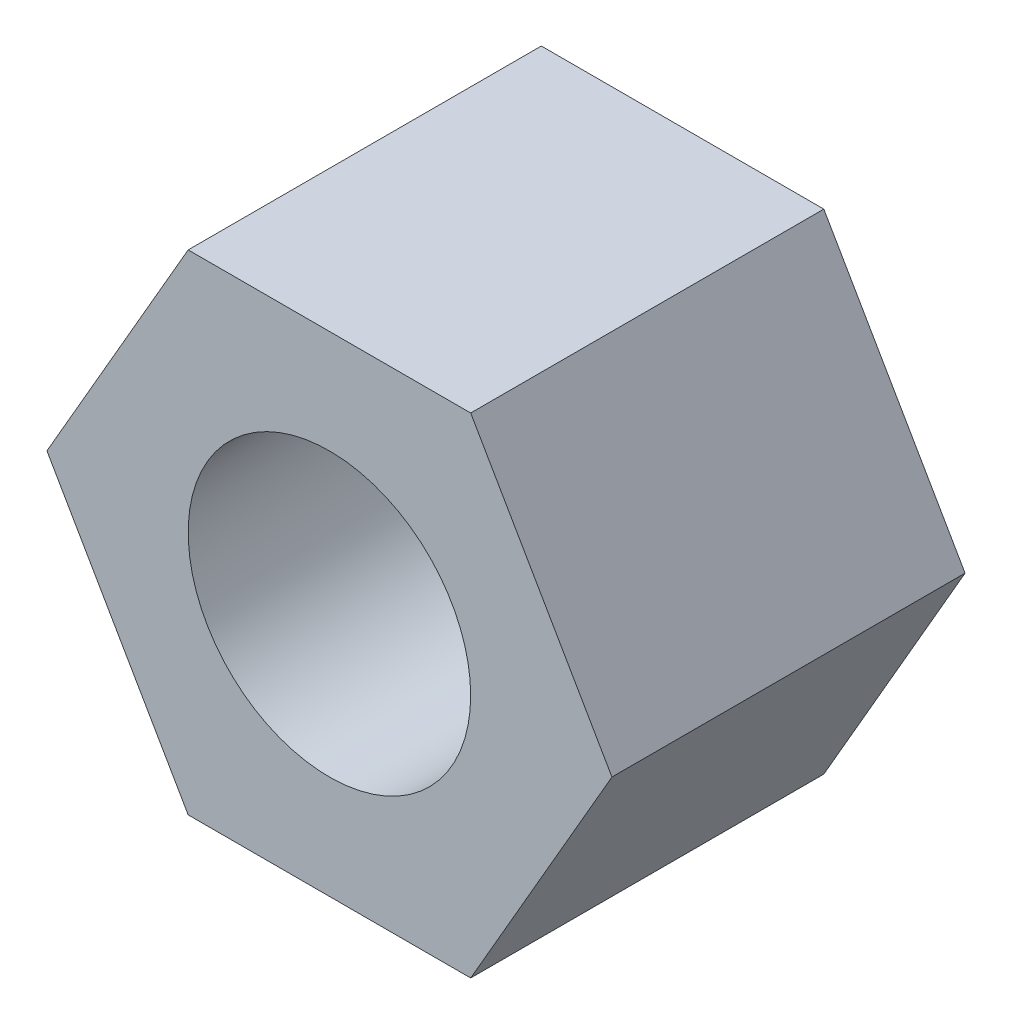
ISO-10303-21;
HEADER;
FILE_DESCRIPTION(('STEP AP214'),'2;1');
FILE_NAME('part.step','',(''),(''),'','','');
FILE_SCHEMA(('AUTOMOTIVE_DESIGN { 1 0 10303 214 1 1 1 1 }'));
ENDSEC;
DATA;
#1=APPLICATION_CONTEXT('core data for automotive mechanical design processes');
#2=APPLICATION_PROTOCOL_DEFINITION('international standard','automotive_design',2000,#1);
#3=PRODUCT_CONTEXT('',#1,'mechanical');
#4=PRODUCT('Part','Part','',(#3));
#5=PRODUCT_RELATED_PRODUCT_CATEGORY('part','',(#4));
#6=PRODUCT_DEFINITION_FORMATION('','',#4);
#7=PRODUCT_DEFINITION_CONTEXT('part definition',#1,'design');
#8=PRODUCT_DEFINITION('design','',#6,#7);
#9=PRODUCT_DEFINITION_SHAPE('','',#8);
#10=(LENGTH_UNIT() NAMED_UNIT(*) SI_UNIT(.MILLI.,.METRE.));
#11=(NAMED_UNIT(*) PLANE_ANGLE_UNIT() SI_UNIT($,.RADIAN.));
#12=(NAMED_UNIT(*) SI_UNIT($,.STERADIAN.) SOLID_ANGLE_UNIT());
#13=UNCERTAINTY_MEASURE_WITH_UNIT(LENGTH_MEASURE(1.E-05),#10,'distance_accuracy_value','');
#14=(GEOMETRIC_REPRESENTATION_CONTEXT(3) GLOBAL_UNCERTAINTY_ASSIGNED_CONTEXT((#13)) GLOBAL_UNIT_ASSIGNED_CONTEXT((#10,
#11,#12)) REPRESENTATION_CONTEXT('',''));
#15=CARTESIAN_POINT('',(0.,0.,0.));
#16=DIRECTION('',(0.,0.,1.));
#17=DIRECTION('',(1.,0.,0.));
#18=AXIS2_PLACEMENT_3D('',#15,#16,#17);
#19=CARTESIAN_POINT('',(0.,0.,15.));
#20=DIRECTION('',(0.,0.,1.));
#21=DIRECTION('',(1.,0.,0.));
#22=AXIS2_PLACEMENT_3D('',#19,#20,#21);
#23=PLANE('',#22);
#24=DIRECTION('',(0.499999999999995,0.866025403784441,0.));
#25=VECTOR('',#24,1.);
#26=CARTESIAN_POINT('',(6.00000000000009,-10.3923048454131,15.));
#27=LINE('',#26,#25);
#28=CARTESIAN_POINT('',(6.00000000000009,-10.3923048454131,15.));
#29=VERTEX_POINT('',#28);
#30=CARTESIAN_POINT('',(11.9999999999999,0.,15.));
#31=VERTEX_POINT('',#30);
#32=EDGE_CURVE('E133',#29,#31,#27,.T.);
#33=ORIENTED_EDGE('',*,*,#32,.T.);
#34=DIRECTION('',(-0.500000000000001,0.866025403784438,0.));
#35=VECTOR('',#34,1.);
#36=CARTESIAN_POINT('',(11.9999999999999,0.,15.));
#37=LINE('',#36,#35);
#38=CARTESIAN_POINT('',(5.99999999999994,10.3923048454132,15.));
#39=VERTEX_POINT('',#38);
#40=EDGE_CURVE('E91',#31,#39,#37,.T.);
#41=ORIENTED_EDGE('',*,*,#40,.T.);
#42=DIRECTION('',(-1.,0.,0.));
#43=VECTOR('',#42,1.);
#44=CARTESIAN_POINT('',(5.99999999999994,10.3923048454132,15.));
#45=LINE('',#44,#43);
#46=CARTESIAN_POINT('',(-6.00000000000001,10.3923048454132,15.));
#47=VERTEX_POINT('',#46);
#48=EDGE_CURVE('E106',#39,#47,#45,.T.);
#49=ORIENTED_EDGE('',*,*,#48,.T.);
#50=DIRECTION('',(-0.499999999999995,-0.866025403784441,0.));
#51=VECTOR('',#50,1.);
#52=CARTESIAN_POINT('',(-6.00000000000001,10.3923048454132,15.));
#53=LINE('',#52,#51);
#54=CARTESIAN_POINT('',(-11.9999999999999,0.,15.));
#55=VERTEX_POINT('',#54);
#56=EDGE_CURVE('E99',#47,#55,#53,.T.);
#57=ORIENTED_EDGE('',*,*,#56,.T.);
#58=DIRECTION('',(0.500000000000007,-0.866025403784435,0.));
#59=VECTOR('',#58,1.);
#60=CARTESIAN_POINT('',(-11.9999999999999,0.,15.));
#61=LINE('',#60,#59);
#62=CARTESIAN_POINT('',(-5.99999999999987,-10.3923048454133,15.));
#63=VERTEX_POINT('',#62);
#64=EDGE_CURVE('E102',#55,#63,#61,.T.);
#65=ORIENTED_EDGE('',*,*,#64,.T.);
#66=DIRECTION('',(1.,0.,0.));
#67=VECTOR('',#66,1.);
#68=CARTESIAN_POINT('',(-5.99999999999987,-10.3923048454133,15.));
#69=LINE('',#68,#67);
#70=EDGE_CURVE('E57',#63,#29,#69,.T.);
#71=ORIENTED_EDGE('',*,*,#70,.T.);
#72=EDGE_LOOP('',(#33,#41,#49,#57,#65,#71));
#73=FACE_BOUND('',#72,.T.);
#74=CARTESIAN_POINT('',(0.,0.,15.));
#75=DIRECTION('',(0.,0.,1.));
#76=DIRECTION('',(1.,0.,0.));
#77=AXIS2_PLACEMENT_3D('',#74,#75,#76);
#78=CIRCLE('',#77,6.);
#79=CARTESIAN_POINT('',(6.,0.,15.));
#80=VERTEX_POINT('',#79);
#81=EDGE_CURVE('E126',#80,#80,#78,.T.);
#82=ORIENTED_EDGE('',*,*,#81,.F.);
#83=EDGE_LOOP('',(#82));
#84=FACE_BOUND('',#83,.T.);
#85=ADVANCED_FACE('F39',(#73,#84),#23,.T.);
#86=CARTESIAN_POINT('',(0.,0.,0.));
#87=DIRECTION('',(0.,0.,1.));
#88=DIRECTION('',(1.,0.,0.));
#89=AXIS2_PLACEMENT_3D('',#86,#87,#88);
#90=PLANE('',#89);
#91=DIRECTION('',(0.499999999999995,0.866025403784441,0.));
#92=VECTOR('',#91,1.);
#93=CARTESIAN_POINT('',(6.00000000000009,-10.3923048454131,0.));
#94=LINE('',#93,#92);
#95=CARTESIAN_POINT('',(6.00000000000009,-10.3923048454131,0.));
#96=VERTEX_POINT('',#95);
#97=CARTESIAN_POINT('',(11.9999999999999,0.,0.));
#98=VERTEX_POINT('',#97);
#99=EDGE_CURVE('E123',#96,#98,#94,.T.);
#100=ORIENTED_EDGE('',*,*,#99,.F.);
#101=DIRECTION('',(1.,0.,0.));
#102=VECTOR('',#101,1.);
#103=CARTESIAN_POINT('',(-5.99999999999987,-10.3923048454133,0.));
#104=LINE('',#103,#102);
#105=CARTESIAN_POINT('',(-5.99999999999987,-10.3923048454133,0.));
#106=VERTEX_POINT('',#105);
#107=EDGE_CURVE('E82',#106,#96,#104,.T.);
#108=ORIENTED_EDGE('',*,*,#107,.F.);
#109=DIRECTION('',(0.500000000000007,-0.866025403784435,0.));
#110=VECTOR('',#109,1.);
#111=CARTESIAN_POINT('',(-11.9999999999999,0.,0.));
#112=LINE('',#111,#110);
#113=CARTESIAN_POINT('',(-11.9999999999999,0.,0.));
#114=VERTEX_POINT('',#113);
#115=EDGE_CURVE('E76',#114,#106,#112,.T.);
#116=ORIENTED_EDGE('',*,*,#115,.F.);
#117=DIRECTION('',(-0.499999999999995,-0.866025403784441,0.));
#118=VECTOR('',#117,1.);
#119=CARTESIAN_POINT('',(-6.00000000000001,10.3923048454132,0.));
#120=LINE('',#119,#118);
#121=CARTESIAN_POINT('',(-6.00000000000001,10.3923048454132,0.));
#122=VERTEX_POINT('',#121);
#123=EDGE_CURVE('E111',#122,#114,#120,.T.);
#124=ORIENTED_EDGE('',*,*,#123,.F.);
#125=DIRECTION('',(-1.,0.,0.));
#126=VECTOR('',#125,1.);
#127=CARTESIAN_POINT('',(5.99999999999994,10.3923048454132,0.));
#128=LINE('',#127,#126);
#129=CARTESIAN_POINT('',(5.99999999999994,10.3923048454132,0.));
#130=VERTEX_POINT('',#129);
#131=EDGE_CURVE('E128',#130,#122,#128,.T.);
#132=ORIENTED_EDGE('',*,*,#131,.F.);
#133=DIRECTION('',(-0.500000000000001,0.866025403784438,0.));
#134=VECTOR('',#133,1.);
#135=CARTESIAN_POINT('',(11.9999999999999,0.,0.));
#136=LINE('',#135,#134);
#137=EDGE_CURVE('E130',#98,#130,#136,.T.);
#138=ORIENTED_EDGE('',*,*,#137,.F.);
#139=EDGE_LOOP('',(#100,#108,#116,#124,#132,#138));
#140=FACE_BOUND('',#139,.T.);
#141=CARTESIAN_POINT('',(0.,0.,0.));
#142=DIRECTION('',(0.,0.,1.));
#143=DIRECTION('',(1.,0.,0.));
#144=AXIS2_PLACEMENT_3D('',#141,#142,#143);
#145=CIRCLE('',#144,6.);
#146=CARTESIAN_POINT('',(6.,0.,0.));
#147=VERTEX_POINT('',#146);
#148=EDGE_CURVE('E229',#147,#147,#145,.T.);
#149=ORIENTED_EDGE('',*,*,#148,.T.);
#150=EDGE_LOOP('',(#149));
#151=FACE_BOUND('',#150,.T.);
#152=ADVANCED_FACE('F145',(#140,#151),#90,.F.);
#153=CARTESIAN_POINT('',(6.00000000000009,-10.3923048454131,15.));
#154=DIRECTION('',(-0.866025403784441,0.499999999999995,0.));
#155=DIRECTION('',(-0.499999999999995,-0.866025403784441,0.));
#156=AXIS2_PLACEMENT_3D('',#153,#154,#155);
#157=PLANE('',#156);
#158=ORIENTED_EDGE('',*,*,#99,.T.);
#159=DIRECTION('',(0.,0.,-1.));
#160=VECTOR('',#159,1.);
#161=CARTESIAN_POINT('',(11.9999999999999,0.,15.));
#162=LINE('',#161,#160);
#163=EDGE_CURVE('E11',#31,#98,#162,.T.);
#164=ORIENTED_EDGE('',*,*,#163,.F.);
#165=ORIENTED_EDGE('',*,*,#32,.F.);
#166=DIRECTION('',(0.,0.,-1.));
#167=VECTOR('',#166,1.);
#168=CARTESIAN_POINT('',(6.00000000000009,-10.3923048454131,15.));
#169=LINE('',#168,#167);
#170=EDGE_CURVE('E118',#29,#96,#169,.T.);
#171=ORIENTED_EDGE('',*,*,#170,.T.);
#172=EDGE_LOOP('',(#158,#164,#165,#171));
#173=FACE_BOUND('',#172,.T.);
#174=ADVANCED_FACE('F41',(#173),#157,.F.);
#175=CARTESIAN_POINT('',(11.9999999999999,0.,15.));
#176=DIRECTION('',(-0.866025403784438,-0.500000000000001,0.));
#177=DIRECTION('',(0.500000000000001,-0.866025403784438,0.));
#178=AXIS2_PLACEMENT_3D('',#175,#176,#177);
#179=PLANE('',#178);
#180=ORIENTED_EDGE('',*,*,#137,.T.);
#181=DIRECTION('',(0.,0.,-1.));
#182=VECTOR('',#181,1.);
#183=CARTESIAN_POINT('',(5.99999999999994,10.3923048454132,15.));
#184=LINE('',#183,#182);
#185=EDGE_CURVE('E48',#39,#130,#184,.T.);
#186=ORIENTED_EDGE('',*,*,#185,.F.);
#187=ORIENTED_EDGE('',*,*,#40,.F.);
#188=ORIENTED_EDGE('',*,*,#163,.T.);
#189=EDGE_LOOP('',(#180,#186,#187,#188));
#190=FACE_BOUND('',#189,.T.);
#191=ADVANCED_FACE('F166',(#190),#179,.F.);
#192=CARTESIAN_POINT('',(5.99999999999994,10.3923048454132,15.));
#193=DIRECTION('',(0.,-1.,0.));
#194=DIRECTION('',(1.,0.,0.));
#195=AXIS2_PLACEMENT_3D('',#192,#193,#194);
#196=PLANE('',#195);
#197=ORIENTED_EDGE('',*,*,#131,.T.);
#198=DIRECTION('',(0.,0.,-1.));
#199=VECTOR('',#198,1.);
#200=CARTESIAN_POINT('',(-6.00000000000001,10.3923048454132,15.));
#201=LINE('',#200,#199);
#202=EDGE_CURVE('E113',#47,#122,#201,.T.);
#203=ORIENTED_EDGE('',*,*,#202,.F.);
#204=ORIENTED_EDGE('',*,*,#48,.F.);
#205=ORIENTED_EDGE('',*,*,#185,.T.);
#206=EDGE_LOOP('',(#197,#203,#204,#205));
#207=FACE_BOUND('',#206,.T.);
#208=ADVANCED_FACE('F143',(#207),#196,.F.);
#209=CARTESIAN_POINT('',(-6.00000000000001,10.3923048454132,15.));
#210=DIRECTION('',(0.866025403784442,-0.499999999999995,0.));
#211=DIRECTION('',(0.499999999999995,0.866025403784442,0.));
#212=AXIS2_PLACEMENT_3D('',#209,#210,#211);
#213=PLANE('',#212);
#214=ORIENTED_EDGE('',*,*,#123,.T.);
#215=DIRECTION('',(0.,0.,-1.));
#216=VECTOR('',#215,1.);
#217=CARTESIAN_POINT('',(-11.9999999999999,0.,15.));
#218=LINE('',#217,#216);
#219=EDGE_CURVE('E112',#55,#114,#218,.T.);
#220=ORIENTED_EDGE('',*,*,#219,.F.);
#221=ORIENTED_EDGE('',*,*,#56,.F.);
#222=ORIENTED_EDGE('',*,*,#202,.T.);
#223=EDGE_LOOP('',(#214,#220,#221,#222));
#224=FACE_BOUND('',#223,.T.);
#225=ADVANCED_FACE('F115',(#224),#213,.F.);
#226=CARTESIAN_POINT('',(-11.9999999999999,0.,15.));
#227=DIRECTION('',(0.866025403784434,0.500000000000007,0.));
#228=DIRECTION('',(-0.500000000000007,0.866025403784435,0.));
#229=AXIS2_PLACEMENT_3D('',#226,#227,#228);
#230=PLANE('',#229);
#231=ORIENTED_EDGE('',*,*,#115,.T.);
#232=DIRECTION('',(0.,0.,-1.));
#233=VECTOR('',#232,1.);
#234=CARTESIAN_POINT('',(-5.99999999999987,-10.3923048454133,15.));
#235=LINE('',#234,#233);
#236=EDGE_CURVE('E117',#63,#106,#235,.T.);
#237=ORIENTED_EDGE('',*,*,#236,.F.);
#238=ORIENTED_EDGE('',*,*,#64,.F.);
#239=ORIENTED_EDGE('',*,*,#219,.T.);
#240=EDGE_LOOP('',(#231,#237,#238,#239));
#241=FACE_BOUND('',#240,.T.);
#242=ADVANCED_FACE('F119',(#241),#230,.F.);
#243=CARTESIAN_POINT('',(-5.99999999999987,-10.3923048454133,15.));
#244=DIRECTION('',(0.,1.,0.));
#245=DIRECTION('',(-1.,0.,0.));
#246=AXIS2_PLACEMENT_3D('',#243,#244,#245);
#247=PLANE('',#246);
#248=ORIENTED_EDGE('',*,*,#107,.T.);
#249=ORIENTED_EDGE('',*,*,#170,.F.);
#250=ORIENTED_EDGE('',*,*,#70,.F.);
#251=ORIENTED_EDGE('',*,*,#236,.T.);
#252=EDGE_LOOP('',(#248,#249,#250,#251));
#253=FACE_BOUND('',#252,.T.);
#254=ADVANCED_FACE('F149',(#253),#247,.F.);
#255=CARTESIAN_POINT('',(0.,0.,15.));
#256=DIRECTION('',(0.,0.,-1.));
#257=DIRECTION('',(-1.,0.,0.));
#258=AXIS2_PLACEMENT_3D('',#255,#256,#257);
#259=CYLINDRICAL_SURFACE('',#258,6.);
#260=ORIENTED_EDGE('',*,*,#81,.T.);
#261=EDGE_LOOP('',(#260));
#262=FACE_BOUND('',#261,.T.);
#263=ORIENTED_EDGE('',*,*,#148,.F.);
#264=EDGE_LOOP('',(#263));
#265=FACE_BOUND('',#264,.T.);
#266=ADVANCED_FACE('F151',(#262,#265),#259,.F.);
#267=CLOSED_SHELL('',(#85,#152,#174,#191,#208,#225,#242,#254,#266));
#268=MANIFOLD_SOLID_BREP('B2',#267);
#269=ADVANCED_BREP_SHAPE_REPRESENTATION('',(#18,#268),#14);
#270=SHAPE_DEFINITION_REPRESENTATION(#9,#269);
ENDSEC;
END-ISO-10303-21;
